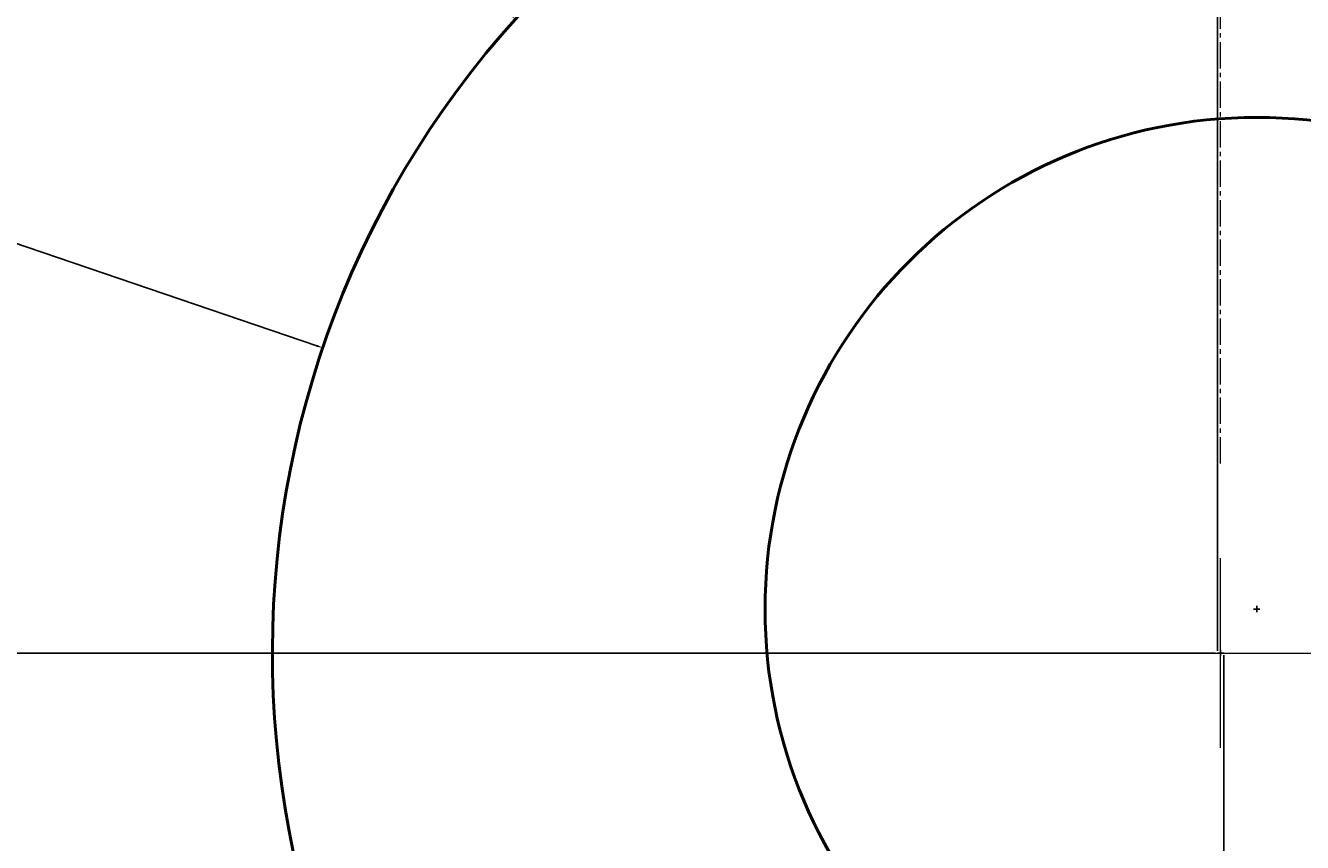
# Model space of a CAD drawing. Units: millimetres. Extents: x -60 to 113, y -37 to 126.
# Tile 13 of 17: x -23 to 13, y 83 to 106. Entities that reach past the tile are written whole.
import ezdxf

# ---------------------------------------------------------------- set-up
doc = ezdxf.new("R2010")
doc.units = ezdxf.units.MM
doc.header["$MEASUREMENT"] = 0
doc.linetypes.add('CENTER2', pattern=[1.125, 0.75, -0.125, 0.125, -0.125])
for name, color, linetype, lineweight in [('M-CNTR', 4, 'CENTER2', 18), ('M-DIMS', 2, 'Continuous', 25), ('M-OUTL', 7, 'Continuous', 50)]:
    doc.layers.add(name, color=color, linetype=linetype, lineweight=lineweight)
doc.styles.get("Standard").update_dxf_attribs({"font": 'arial.ttf'})
doc.dimstyles.get("Standard").update_dxf_attribs({"dimtxt": 0.18, "dimasz": 0.18, "dimexe": 0.18, "dimexo": 0.0625, "dimgap": 0.09, "dimtad": 0, "dimtih": 1, "dimtoh": 1, "dimdec": 4, "dimzin": 0, "dimdsep": 46, "dimtxsty": 'Standard', "dimcen": 0.09, "dimadec": 0, "dimazin": 0, "dimtfac": 1, "dimtdec": 4, "dimtofl": 0, "dimtmove": 0, "dimatfit": 3, "dimfxl": 1, "dimtolj": 1, "dimtzin": 0, "dimarcsym": 0})

# ---------------------------------------------------------------- blocks, each defined once
blk = doc.blocks.new('*U1')
at = {"layer": 'M-CNTR', "color": 0, "transparency": 16777216}
for p, q in [((0, 5.4), (0, 27.12)), ((-27.12, 0), (-5.4, 0))]:
    blk.add_line(p, q, dxfattribs=at)
at = {"layer": 'M-CNTR', "color": 0, "linetype": 'Continuous', "transparency": 16777216}
for p, q in [((0, -2.7), (0, 2.7)), ((-2.7, 0), (2.7, 0))]:
    blk.add_line(p, q, dxfattribs=at)
blk = doc.blocks.new('*D4')
at = {"layer": 'Defpoints', "color": 0, "transparency": 16777216}
for p in [(-14.94, 97.225), (10.622, 88.533)]:
    blk.add_point(p, dxfattribs=at)
at = {"layer": 'M-DIMS', "color": 0, "lineweight": -2, "transparency": 16777216}
for p, q in [((-37.421, 104.807), (-37.241, 104.807)), ((-37.241, 104.807), (-15.111, 97.283)), ((10.532, 88.533), (10.712, 88.533)), ((10.622, 88.443), (10.622, 88.623))]:
    blk.add_line(p, q, dxfattribs=at)
at = {"layer": 'M-DIMS', "color": 0, "transparency": 16777216}
blk.add_solid([(-15.101, 97.311), (-15.12, 97.254), (-14.94, 97.225)], dxfattribs=at)
at = {"layer": 'M-DIMS', "color": 0, "transparency": 16777216, "insert": (-39.9, 104.807), "char_height": 0.18, "attachment_point": 5}
blk.add_mtext('\\A1;{\\H11.11111x;R27}', dxfattribs=at)
blk = doc.blocks.new('*D8')
at = {"layer": 'Defpoints', "color": 0, "transparency": 16777216}
for p in [(23.977, 96.423), (-0.678, 83.151)]:
    blk.add_point(p, dxfattribs=at)
at = {"layer": 'M-DIMS', "color": 0, "lineweight": -2, "transparency": 16777216}
for p, q in [((48.912, 109.846), (24.135, 96.508)), ((49.092, 109.846), (48.912, 109.846)), ((11.649, 89.697), (11.649, 89.877)), ((11.559, 89.787), (11.739, 89.787))]:
    blk.add_line(p, q, dxfattribs=at)
at = {"layer": 'M-DIMS', "color": 0, "transparency": 16777216}
blk.add_solid([(24.121, 96.535), (24.149, 96.482), (23.977, 96.423)], dxfattribs=at)
at = {"layer": 'M-DIMS', "color": 0, "transparency": 16777216, "insert": (51.704, 109.846), "char_height": 0.18, "attachment_point": 5}
blk.add_mtext('\\A1;{\\H11.11111x;%%C28}', dxfattribs=at)
blk = doc.blocks.new('*D12')
at = {"layer": 'Defpoints', "color": 0, "transparency": 16777216}
for p in [(10.532, 88.533), (-58.719, 6.903), (11.329, 6.903)]:
    blk.add_point(p, dxfattribs=at)
at = {"layer": 'M-DIMS', "color": 0, "lineweight": -2, "transparency": 16777216}
for p, q in [((10.47, 88.533), (-58.899, 88.533)), ((-58.719, 88.353), (-58.719, 48.829)), ((-58.719, 7.083), (-58.719, 46.607)), ((11.267, 6.903), (-58.899, 6.903))]:
    blk.add_line(p, q, dxfattribs=at)
at = {"layer": 'M-DIMS', "color": 0, "transparency": 16777216}
for points in [[(-58.749, 88.353), (-58.689, 88.353), (-58.719, 88.533)], [(-58.749, 7.083), (-58.689, 7.083), (-58.719, 6.903)]]:
    blk.add_solid(points, dxfattribs=at)
at = {"layer": 'M-DIMS', "color": 0, "transparency": 16777216, "insert": (-58.719, 47.718), "char_height": 0.18, "attachment_point": 5}
blk.add_mtext('\\A1;{\\H11.11111x;82}', dxfattribs=at)
blk = doc.blocks.new('*D16')
at = {"layer": 'Defpoints', "color": 0, "transparency": 16777216}
for p in [(10.712, 88.533), (10.712, 88.533), (10.712, 6.442)]:
    blk.add_point(p, dxfattribs=at)
at = {"layer": 'M-DIMS', "color": 0, "lineweight": -2, "transparency": 16777216}
for p, q in [((10.712, 88.47), (10.712, 6.262)), ((10.712, 88.47), (10.712, 6.262)), ((10.532, 6.442), (10.352, 6.442)), ((10.892, 6.442), (11.072, 6.442))]:
    blk.add_line(p, q, dxfattribs=at)
at = {"layer": 'M-DIMS', "color": 0, "transparency": 16777216}
for points in [[(10.532, 6.472), (10.532, 6.412), (10.712, 6.442)], [(10.892, 6.472), (10.892, 6.412), (10.712, 6.442)]]:
    blk.add_solid(points, dxfattribs=at)
at = {"layer": 'M-DIMS', "color": 0, "transparency": 16777216, "insert": (11.536, 6.442), "char_height": 0.18, "attachment_point": 5}
blk.add_mtext('\\A1;0.0000', dxfattribs=at)
blk = doc.blocks.new('*D17')
at = {"layer": 'Defpoints', "color": 0, "transparency": 16777216}
for p in [(67.355, 124.823), (10.532, 88.533), (67.355, 6.442)]:
    blk.add_point(p, dxfattribs=at)
at = {"layer": 'M-DIMS', "color": 0, "lineweight": -2, "transparency": 16777216}
for p, q in [((10.532, 88.595), (10.532, 125.003)), ((10.712, 124.823), (37.422, 124.823)), ((67.175, 124.823), (40.465, 124.823)), ((67.355, 6.504), (67.355, 125.003))]:
    blk.add_line(p, q, dxfattribs=at)
at = {"layer": 'M-DIMS', "color": 0, "transparency": 16777216}
for points in [[(10.712, 124.853), (10.712, 124.793), (10.532, 124.823)], [(67.175, 124.853), (67.175, 124.793), (67.355, 124.823)]]:
    blk.add_solid(points, dxfattribs=at)
at = {"layer": 'M-DIMS', "color": 0, "transparency": 16777216, "insert": (38.944, 124.823), "char_height": 0.18, "attachment_point": 5}
blk.add_mtext('\\A1;{\\H11.11111x;56}', dxfattribs=at)
blk = doc.blocks.new('HOLE-D28')
blk.add_circle((14, 14), 14)
blk = doc.blocks.new('*D20')
at = {"layer": 'Defpoints', "color": 0, "transparency": 16777216}
for p in [(-9.458, 106.582), (10.622, 88.533)]:
    blk.add_point(p, dxfattribs=at)
at = {"layer": 'M-DIMS', "color": 0, "lineweight": -2, "transparency": 16777216}
for p, q in [((-21.686, 117.412), (-21.506, 117.412)), ((-21.506, 117.412), (-9.592, 106.703)), ((10.532, 88.533), (10.712, 88.533)), ((10.622, 88.443), (10.622, 88.623))]:
    blk.add_line(p, q, dxfattribs=at)
at = {"layer": 'M-DIMS', "color": 0, "transparency": 16777216}
blk.add_solid([(-9.572, 106.725), (-9.612, 106.68), (-9.458, 106.582)], dxfattribs=at)
at = {"layer": 'M-DIMS', "color": 0, "transparency": 16777216, "insert": (-22.499, 117.412), "char_height": 0.18, "attachment_point": 5}
blk.add_mtext('\\A1;3X R27.0000', dxfattribs=at)
blk = doc.blocks.new('*D24')
at = {"layer": 'Defpoints', "color": 0, "transparency": 16777216}
for p in [(48.596, 76.851), (-30.775, 49.351)]:
    blk.add_point(p, dxfattribs=at)
at = {"layer": 'M-DIMS', "color": 0, "lineweight": -2, "transparency": 16777216}
for p, q in [((96.218, 93.35), (48.766, 76.909)), ((96.398, 93.35), (96.218, 93.35)), ((-30.865, 49.351), (-30.685, 49.351)), ((-30.775, 49.261), (-30.775, 49.441))]:
    blk.add_line(p, q, dxfattribs=at)
at = {"layer": 'M-DIMS', "color": 0, "transparency": 16777216}
blk.add_solid([(48.756, 76.938), (48.776, 76.881), (48.596, 76.851)], dxfattribs=at)
at = {"layer": 'M-DIMS', "color": 0, "transparency": 16777216, "insert": (97.018, 93.35), "char_height": 0.18, "attachment_point": 5}
blk.add_mtext('\\A1;R84.0000', dxfattribs=at)

msp = doc.modelspace()

# ---------------------------------------------------------------- linework, layer by layer
at = {"layer": 'M-OUTL'}
msp.add_arc((10.62227, 88.53289), 27, 43.425324, 223.425324, dxfattribs=at)

# ---------------------------------------------------------------- block references
at = {"layer": 'M-CNTR'}
msp.add_blockref('*U1', (10.62227, 88.53289), dxfattribs=at)
at = {"layer": 'M-OUTL'}
msp.add_blockref('HOLE-D28', (-2.3502, 75.7872), dxfattribs=at)

# ---------------------------------------------------------------- dimensions: what is measured, and where the dimension line sits
at = {"layer": 'M-DIMS'}
dim = msp.add_linear_dim(base=(67.35481, 124.82251), p1=(10.53227, 88.53289), p2=(67.35481, 6.44179), text='{\\H11.11111x;56}', dimstyle='Standard', override={"dimclrd": 0, "dimclre": 0, "dimclrt": 0}, dxfattribs=at)
dim.commit()
dim.dimension.update_dxf_attribs({"geometry": '*D17', "text_midpoint": (38.94354, 124.82251)})
for mpoint, text, override, picture, middle in [((-9.45794, 106.58241), '3X <>', {"dimdec": 4, "dimlfac": 1, "dimrnd": 0, "dimzin": 0, "dimdsep": 46, "dimlunit": 2}, '*D20', (-22.49876, 117.41213)), ((-14.94042, 97.22479), '{\\H11.11111x;R27}', {"dimclrd": 0, "dimclre": 0, "dimclrt": 0}, '*D4', (-39.9004, 104.80746))]:
    dim = msp.add_radius_dim(center=(10.62227, 88.53289), mpoint=mpoint, text=text, dimstyle='Standard', override=override, dxfattribs=at)
    dim.commit()
    dim.dimension.update_dxf_attribs({"geometry": picture, "text_midpoint": middle, "dimtype": 164})
dim = msp.add_diameter_dim_2p(p1=(-0.67791, 83.1508), p2=(23.97668, 96.423), text='{\\H11.11111x;%%C28}', dimstyle='Standard', override={"dimclrd": 0, "dimclre": 0, "dimclrt": 0}, dxfattribs=at)
dim.commit()
dim.dimension.update_dxf_attribs({"geometry": '*D8', "text_midpoint": (51.70419, 109.84614), "dimtype": 163})
dim = msp.add_radius_dim(center=(-30.77517, 49.3506), mpoint=(48.59582, 76.85052), dimstyle='Standard', override={"dimdec": 4, "dimlfac": 1, "dimrnd": 0, "dimzin": 0, "dimdsep": 46, "dimlunit": 2}, dxfattribs=at)
dim.commit()
dim.dimension.update_dxf_attribs({"geometry": '*D24', "text_midpoint": (97.01779, 93.35047), "dimtype": 164})
dim = msp.add_linear_dim(base=(-58.71857, 6.9027), p1=(10.53227, 88.53289), p2=(11.32938, 6.9027), angle=90, text='{\\H11.11111x;82}', dimstyle='Standard', override={"dimclrd": 0, "dimclre": 0, "dimclrt": 0}, dxfattribs=at)
dim.commit()
dim.dimension.update_dxf_attribs({"geometry": '*D12', "text_midpoint": (-58.71857, 47.71779)})
dim = msp.add_linear_dim(base=(10.712269814, 6.441792179), p1=(10.712269814, 88.5328900903), p2=(10.712269814, 88.5328900903), dimstyle='Standard', override={"dimclrd": 0, "dimclre": 0, "dimclrt": 0}, dxfattribs=at)
dim.commit()
dim.dimension.update_dxf_attribs({"geometry": '*D16', "text_midpoint": (11.5355917785, 6.441792179)})

doc.saveas('drawing.dxf')
